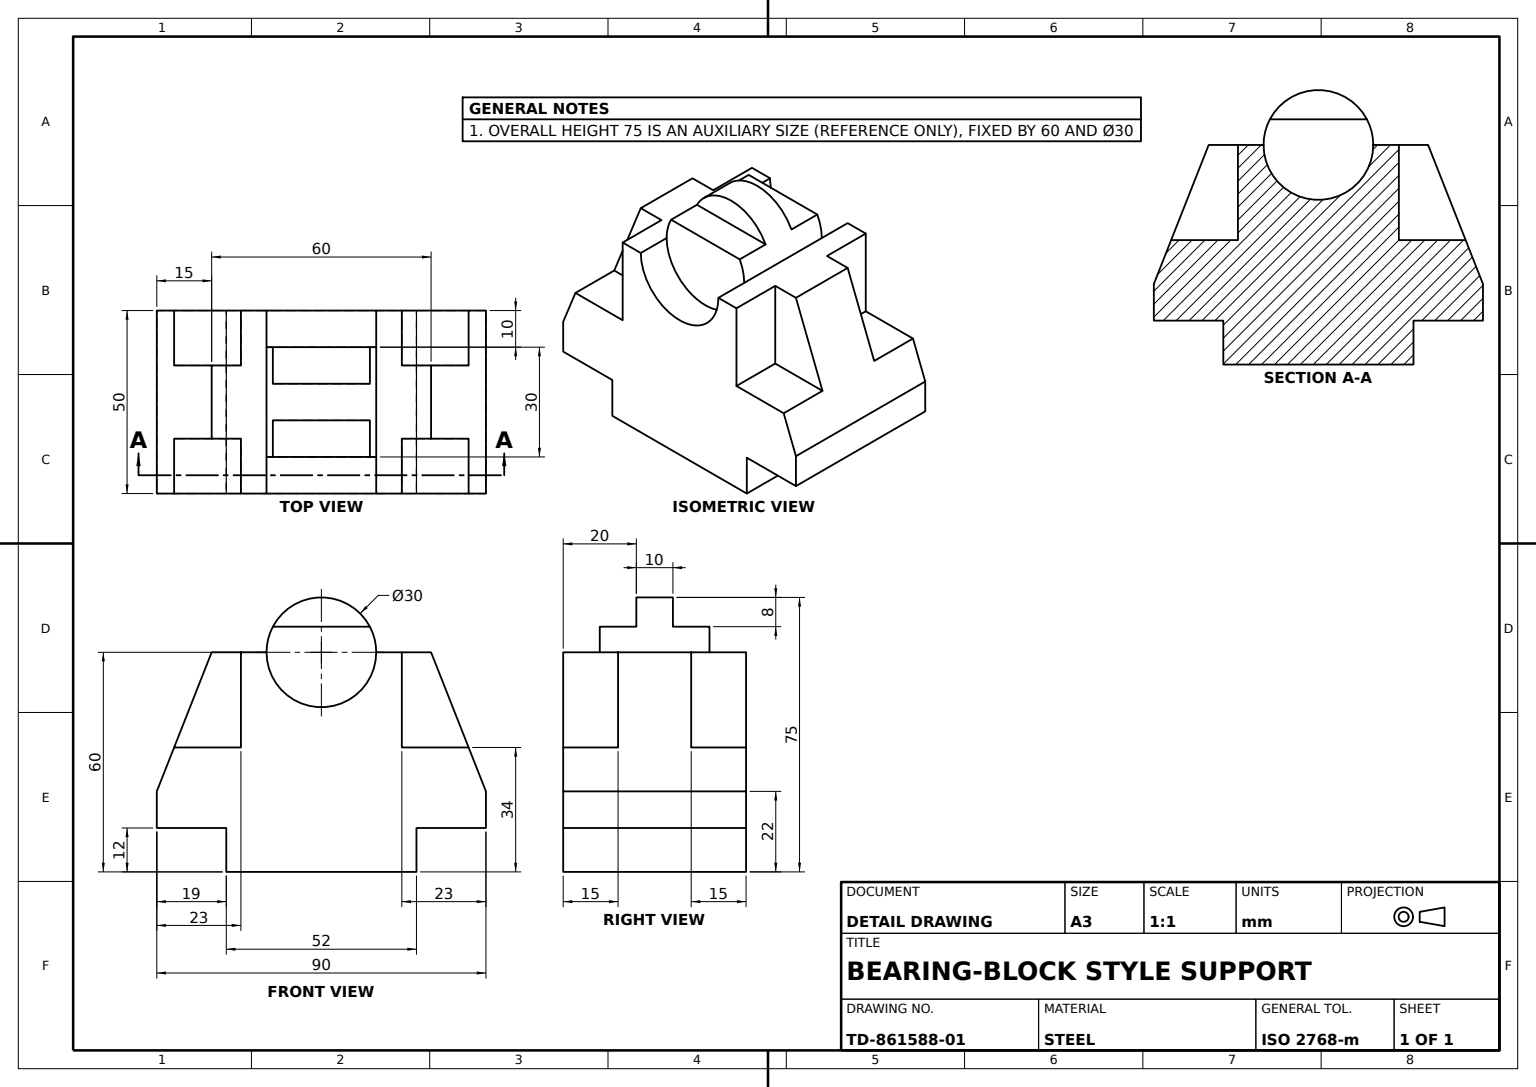
SolidWorks part; units mm, degrees
material "Plain Carbon Steel"
ref_plane "Front Plane" through (0, 0, 0) normal (0, 0, 1) x (1, 0, 0)
ref_plane "Top Plane" through (0, 0, 0) normal (0, 1, 0) x (1, 0, 0)
ref_plane "Right Plane" through (0, 0, 0) normal (1, 0, 0) x (0, 0, -1)
sketch "Saddle Profile Sketch" plane through (0, 0, 0) normal (0, 0, 1) x (1, 0, 0)
  line L0 (-45, 0) -> (-45, 10)
  line L1 (-45, 10) -> (-30, 48)
  line L7 (30, 48) -> (45, 10)
  line L8 (45, 10) -> (45, 0)
  line L10 (26, 0) -> (26, -12)
  line L11 (26, -12) -> (-26, -12)
  line L12 (-26, -12) -> (-26, 0)
  line L13 (-26, 0) -> (-45, 0)
  line L14 (26, 0) -> (45, 0)
  line L15 (45, 0) -> (45, 10)
  line L16 (0, -12) -> (0, 0) construction
  line L17 (-30, 48) -> (30, 48)
  point P2 (0, -12)
  point P4 (0, 48)
  dimension "D1" = 52
  dimension "D2" = 12
  dimension "D3" = 10
  dimension "D4" = 90
  dimension "D5" = 60
  dimension "D6" = 60
extrude "Saddle Body" add sketch "Saddle Profile Sketch" along normal mid plane 50
sketch "Corner Pocket Sketch" plane through (0, 0, 25) normal (0, 0, 1) x (1, 0, 0)
  line L0 (-30, 48) -> (-22, 48)
  line L1 (-30, 48) -> (30, 48) construction
  line L2 (-22, 48) -> (-22, 22)
  line L3 (-22, 22) -> (-40.2632, 22)
  line L4 (-45, 10) -> (-30, 48) construction
  line L5 (-40.2632, 22) -> (-30, 48)
  line L6 (26, -12) -> (-26, -12) construction
  dimension "D1" = 34
  dimension "D2" = 22
extrude "Corner Pocket 34x22" cut sketch "Corner Pocket Sketch" against normal blind 15
mirror "Corner Pocket Mirror Front" about plane through (0, 0, 0) normal (0, 0, 1) of "Corner Pocket 34x22"
mirror "Corner Pocket Mirror Side" about plane through (0, 0, 0) normal (1, 0, 0) of "Corner Pocket Mirror Front", "Corner Pocket 34x22"
sketch "Bore Sketch" plane through (0, 0, 25) normal (0, 0, 1) x (1, 0, 0)
  line L0 (-22, 48) -> (22, 48) construction
  circle A0 centre (0, 48) radius 15
  dimension "D1" = 30
extrude "Bore Ø30" cut sketch "Bore Sketch" against normal through all
sketch "Bore Plug Sketch" plane through (0, 0, 0) normal (0, 0, 1) x (1, 0, 0)
  circle A0 centre (0, 48) radius 15
  arc A1 (-15, 48) -> (15, 48) centre (0, 48) ccw construction
extrude "Bore Plug" add sketch "Bore Plug Sketch" along normal mid plane 30
sketch "Plug Slot Sketch" plane through (0, 0, 0) normal (1, 0, 0) x (0, 0, -1)
  line L0 (15, 55) -> (5, 55)
  line L1 (15, 48) -> (15, 63) construction
  line L2 (5, 55) -> (5, 63)
  line L3 (15, 63) -> (-15, 63) construction
  line L4 (5, 63) -> (15, 63)
  line L5 (15, 63) -> (15, 55)
  dimension "D1" = 8
  dimension "D2" = 10
extrude "Plug Slot 8x10" cut sketch "Plug Slot Sketch" against normal mid plane 30
mirror "Plug Slot Mirror" about plane through (0, 0, 0) normal (0, 0, 1) of "Plug Slot 8x10"
